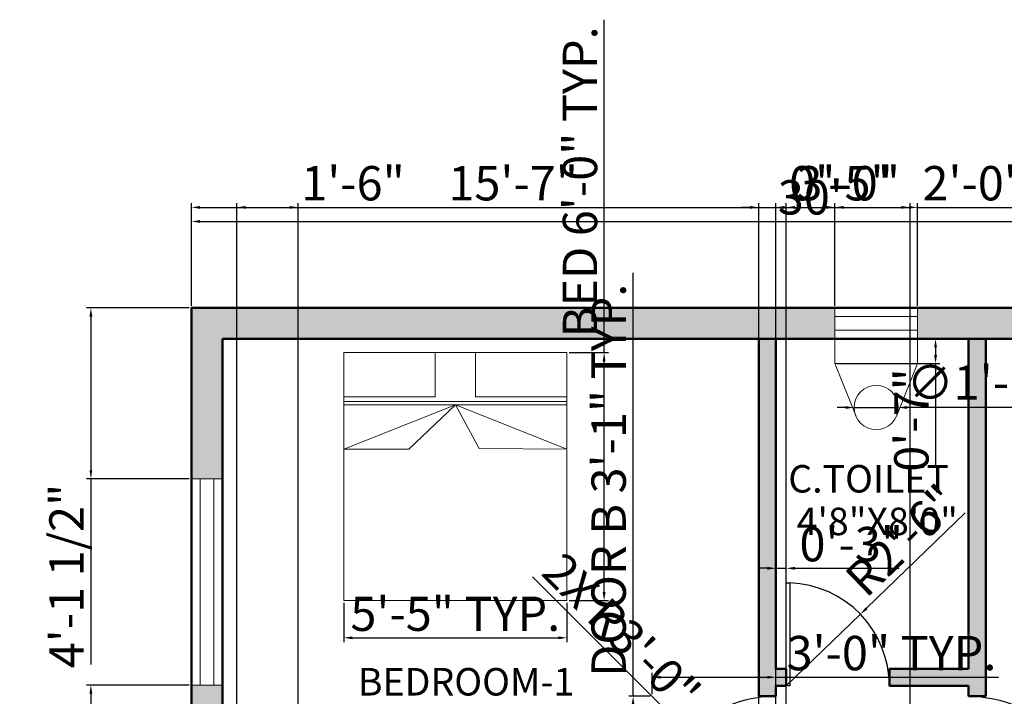
# Model space of a CAD drawing. Units: inches. Extents: x 2719 to 3167, y 1639 to 2327.
# Tile 3 of 4: x 2719 to 3005, y 2130 to 2327. Entities that reach past the tile are written whole.
import ezdxf

# ---------------------------------------------------------------- set-up
doc = ezdxf.new("R2010")
doc.units = ezdxf.units.IN
for name, color, linetype, lineweight in [('A-ANNO-DIMS', 121, 'Continuous', 18), ('A-AREA-IDEN', 121, 'Continuous', 18), ('A-DOOR', 50, 'Continuous', 25), ('A-FLOR-FIXT', 211, 'Continuous', 18), ('A-FURN', 211, 'Continuous', 18), ('A-GLAZ', 191, 'Continuous', 18), ('A-WALL', 7, 'Continuous', 50)]:
    doc.layers.add(name, color=color, linetype=linetype, lineweight=lineweight)
doc.layers.add('A-WALL-PATT', color=251, linetype='Continuous', lineweight=13, true_color=0x636466)
doc.styles.get("Standard").update_dxf_attribs({"font": 'arial.ttf'})
doc.dimstyles.new('ISO-25', dxfattribs={"dimtxt": 10, "dimasz": 2.5, "dimexe": 1.25, "dimexo": 0.625, "dimtad": 1, "dimdec": 0, "dimlunit": 3, "dimtxsty": 'Standard', "dimcen": 2.5, "dimadec": 0, "dimazin": 0, "dimtfac": 1, "dimtdec": 0, "dimtmove": 0, "dimatfit": 3, "dimfxl": 1, "dimarcsym": 0})

# ---------------------------------------------------------------- blocks, each defined once
blk = doc.blocks.new('*D1')
at = {"layer": 'A-ANNO-DIMS', "color": 0, "lineweight": -2, "transparency": 16777216}
for p, q in [((2768.8, 2244.06), (2768.8, 2269.84)), ((2771.3, 2268.59), (3126.3, 2268.59)), ((3128.8, 2244.06), (3128.8, 2269.84))]:
    blk.add_line(p, q, dxfattribs=at)
at = {"layer": 'A-ANNO-DIMS', "color": 0, "transparency": 16777216}
for points in [[(2771.3, 2269.01), (2771.3, 2268.17), (2768.8, 2268.59)], [(3126.3, 2269.01), (3126.3, 2268.17), (3128.8, 2268.59)]]:
    blk.add_solid(points, dxfattribs=at)
at = {"layer": 'Defpoints', "color": 0, "transparency": 16777216}
for p in [(3128.8, 2268.59), (2768.8, 2243.44), (3128.8, 2243.44)]:
    blk.add_point(p, dxfattribs=at)
at = {"layer": 'A-ANNO-DIMS', "color": 0, "transparency": 16777216, "insert": (2948.8, 2274.32), "char_height": 10, "attachment_point": 5}
blk.add_mtext("30'", dxfattribs=at)
blk = doc.blocks.new('BED-DOUBLE')
for p, q in [((0, 57.96), (64.91, 57.96)), ((0, 56.96), (64.91, 56.96)), ((32.46, 56.96), (0, 44.1)), ((32.46, 56.96), (18.94, 44.05)), ((32.46, 56.96), (64.91, 44.04)), ((32.46, 56.96), (39.4, 44.29)), ((18.94, 44.05), (0, 44.05)), ((39.4, 44.29), (64.91, 44.04))]:
    blk.add_line(p, q)
for points in [[(0, 72.15), (64.91, 72.15), (64.91, 0), (0, 0)], [(0, 72.15), (26.55, 72.15), (26.55, 59.27), (0, 59.27)], [(38.37, 72.15), (64.91, 72.15), (64.91, 59.27), (38.37, 59.27)]]:
    blk.add_lwpolyline(points, close=True)
blk = doc.blocks.new('WIN-60IN')
for p, q in [((9, 60), (0, 60)), ((2.5, 60), (2.5, 0)), ((6.5, 60), (6.5, 0)), ((9, 0), (0, 0))]:
    blk.add_line(p, q)
blk = doc.blocks.new('DOOR-36IN-QUARTER-SWING')
for p, q in [((0, 0), (0, 1)), ((0, 1), (36, 1)), ((36, 0), (0, 0)), ((36, 1), (36, 0))]:
    blk.add_line(p, q)
blk.add_arc((36, 1), 36, 90, 180)
blk = doc.blocks.new('*D9')
at = {"layer": 'A-ANNO-DIMS', "color": 0, "lineweight": -2, "transparency": 16777216}
for p, q in [((2888.82, 2230.43), (2888.82, 2327.3)), ((2878.63, 2230.43), (2890.07, 2230.43)), ((2888.82, 2160.78), (2888.82, 2227.93)), ((2878.63, 2158.28), (2890.07, 2158.28))]:
    blk.add_line(p, q, dxfattribs=at)
at = {"layer": 'A-ANNO-DIMS', "color": 0, "transparency": 16777216}
for points in [[(2888.41, 2227.93), (2889.24, 2227.93), (2888.82, 2230.43)], [(2888.41, 2160.78), (2889.24, 2160.78), (2888.82, 2158.28)]]:
    blk.add_solid(points, dxfattribs=at)
at = {"layer": 'Defpoints', "color": 0, "transparency": 16777216}
for p in [(2878, 2230.43), (2888.82, 2230.43), (2878, 2158.28)]:
    blk.add_point(p, dxfattribs=at)
at = {"layer": 'A-ANNO-DIMS', "color": 0, "transparency": 16777216, "insert": (2883.09, 2280.11), "char_height": 10, "attachment_point": 5, "rotation": 90}
blk.add_mtext('BED 6\'-0" TYP.', dxfattribs=at)
blk = doc.blocks.new('*D10')
at = {"layer": 'A-ANNO-DIMS', "color": 0, "lineweight": -2, "transparency": 16777216}
for p, q in [((2813.09, 2157.65), (2813.09, 2146.21)), ((2878, 2157.65), (2878, 2146.21)), ((2815.59, 2147.46), (2875.5, 2147.46))]:
    blk.add_line(p, q, dxfattribs=at)
at = {"layer": 'A-ANNO-DIMS', "color": 0, "transparency": 16777216}
for points in [[(2815.59, 2147.87), (2815.59, 2147.04), (2813.09, 2147.46)], [(2875.5, 2147.87), (2875.5, 2147.04), (2878, 2147.46)]]:
    blk.add_solid(points, dxfattribs=at)
at = {"layer": 'Defpoints', "color": 0, "transparency": 16777216}
for p in [(2813.09, 2158.28), (2878, 2158.28), (2878, 2147.46)]:
    blk.add_point(p, dxfattribs=at)
at = {"layer": 'A-ANNO-DIMS', "color": 0, "transparency": 16777216, "insert": (2845.54, 2153.17), "char_height": 10, "attachment_point": 5}
blk.add_mtext('5\'-5" TYP.', dxfattribs=at)
blk = doc.blocks.new('*D13')
at = {"layer": 'A-ANNO-DIMS', "color": 0, "lineweight": -2, "transparency": 16777216}
for p, q in [((2897.25, 2130.44), (2897.25, 2253.63)), ((2902.17, 2130.44), (2896, 2130.44)), ((2897.25, 2095.94), (2897.25, 2127.94)), ((2902.17, 2093.44), (2896, 2093.44))]:
    blk.add_line(p, q, dxfattribs=at)
at = {"layer": 'A-ANNO-DIMS', "color": 0, "transparency": 16777216}
for points in [[(2896.83, 2127.94), (2897.66, 2127.94), (2897.25, 2130.44)], [(2896.83, 2095.94), (2897.66, 2095.94), (2897.25, 2093.44)]]:
    blk.add_solid(points, dxfattribs=at)
at = {"layer": 'Defpoints', "color": 0, "transparency": 16777216}
for p in [(2897.25, 2130.44), (2902.8, 2130.44), (2902.8, 2093.44)]:
    blk.add_point(p, dxfattribs=at)
at = {"layer": 'A-ANNO-DIMS', "color": 0, "transparency": 16777216, "insert": (2891.44, 2193.29), "char_height": 10, "attachment_point": 5, "rotation": 90}
blk.add_mtext('DOOR B 3\'-1" TYP.', dxfattribs=at)
blk = doc.blocks.new('*D14')
at = {"layer": 'A-ANNO-DIMS', "color": 0, "lineweight": -2, "transparency": 16777216}
for p, q in [((2902.8, 2131.06), (2902.8, 2137.24)), ((2938.8, 2131.06), (2938.8, 2137.24)), ((2905.3, 2135.99), (2936.3, 2135.99)), ((2938.8, 2135.99), (3003.49, 2135.99))]:
    blk.add_line(p, q, dxfattribs=at)
at = {"layer": 'A-ANNO-DIMS', "color": 0, "transparency": 16777216}
for points in [[(2905.3, 2136.4), (2905.3, 2135.57), (2902.8, 2135.99)], [(2936.3, 2136.4), (2936.3, 2135.57), (2938.8, 2135.99)]]:
    blk.add_solid(points, dxfattribs=at)
at = {"layer": 'Defpoints', "color": 0, "transparency": 16777216}
for p in [(2938.8, 2135.99), (2902.8, 2130.44), (2938.8, 2130.44)]:
    blk.add_point(p, dxfattribs=at)
at = {"layer": 'A-ANNO-DIMS', "color": 0, "transparency": 16777216, "insert": (2972.4, 2141.72), "char_height": 10, "attachment_point": 5}
blk.add_mtext('3\'-0" TYP.', dxfattribs=at)
blk = doc.blocks.new('*D17')
at = {"layer": 'A-ANNO-DIMS', "color": 0, "lineweight": -2, "transparency": 16777216}
for p, q in [((2768.8, 2244.06), (2768.8, 2273.94)), ((2955.97, 2244.06), (2955.97, 2273.94)), ((2771.3, 2272.69), (2953.47, 2272.69))]:
    blk.add_line(p, q, dxfattribs=at)
at = {"layer": 'A-ANNO-DIMS', "color": 0, "transparency": 16777216}
for points in [[(2771.3, 2273.1), (2771.3, 2272.27), (2768.8, 2272.69)], [(2953.47, 2273.1), (2953.47, 2272.27), (2955.97, 2272.69)]]:
    blk.add_solid(points, dxfattribs=at)
at = {"layer": 'Defpoints', "color": 0, "transparency": 16777216}
for p in [(2955.97, 2272.69), (2768.8, 2243.44), (2955.97, 2243.44)]:
    blk.add_point(p, dxfattribs=at)
at = {"layer": 'A-ANNO-DIMS', "color": 0, "transparency": 16777216, "insert": (2862.38, 2278.42), "char_height": 10, "attachment_point": 5}
blk.add_mtext('15\'-7"', dxfattribs=at)
blk = doc.blocks.new('*D18')
at = {"layer": 'A-ANNO-DIMS', "color": 0, "lineweight": -2, "transparency": 16777216}
for p, q in [((2955.97, 2244.06), (2955.97, 2273.94)), ((2979.97, 2244.06), (2979.97, 2273.94)), ((2958.47, 2272.69), (2977.47, 2272.69)), ((2979.97, 2272.69), (3010.48, 2272.69))]:
    blk.add_line(p, q, dxfattribs=at)
at = {"layer": 'A-ANNO-DIMS', "color": 0, "transparency": 16777216}
for points in [[(2958.47, 2273.1), (2958.47, 2272.27), (2955.97, 2272.69)], [(2977.47, 2273.1), (2977.47, 2272.27), (2979.97, 2272.69)]]:
    blk.add_solid(points, dxfattribs=at)
at = {"layer": 'Defpoints', "color": 0, "transparency": 16777216}
for p in [(2979.97, 2272.69), (2955.97, 2243.44), (2979.97, 2243.44)]:
    blk.add_point(p, dxfattribs=at)
at = {"layer": 'A-ANNO-DIMS', "color": 0, "transparency": 16777216, "insert": (2996.48, 2278.42), "char_height": 10, "attachment_point": 5}
blk.add_mtext('2\'-0"', dxfattribs=at)
blk = doc.blocks.new('*D19')
at = {"layer": 'A-ANNO-DIMS', "color": 0, "lineweight": -2, "transparency": 16777216}
for p, q in [((2768.17, 2243.44), (2738.3, 2243.44)), ((2739.55, 2240.94), (2739.55, 2196.22)), ((2768.17, 2193.72), (2738.3, 2193.72)), ((2739.55, 2193.72), (2739.55, 2139.68))]:
    blk.add_line(p, q, dxfattribs=at)
at = {"layer": 'A-ANNO-DIMS', "color": 0, "transparency": 16777216}
for points in [[(2739.13, 2240.94), (2739.96, 2240.94), (2739.55, 2243.44)], [(2739.13, 2196.22), (2739.96, 2196.22), (2739.55, 2193.72)]]:
    blk.add_solid(points, dxfattribs=at)
at = {"layer": 'Defpoints', "color": 0, "transparency": 16777216}
for p in [(2768.8, 2243.44), (2739.55, 2193.72), (2768.8, 2193.72)]:
    blk.add_point(p, dxfattribs=at)
at = {"layer": 'A-ANNO-DIMS', "color": 0, "transparency": 16777216, "insert": (2733.75, 2165.45), "char_height": 10, "attachment_point": 5, "rotation": 90}
blk.add_mtext('4\'-1 1/2"', dxfattribs=at)
blk = doc.blocks.new('*D20')
at = {"layer": 'A-ANNO-DIMS', "color": 0, "lineweight": -2, "transparency": 16777216}
for p, q in [((2768.17, 2133.72), (2738.3, 2133.72)), ((2739.55, 2131.22), (2739.55, 2064.55)), ((2768.17, 2062.05), (2738.3, 2062.05))]:
    blk.add_line(p, q, dxfattribs=at)
at = {"layer": 'A-ANNO-DIMS', "color": 0, "transparency": 16777216}
for points in [[(2739.13, 2131.22), (2739.96, 2131.22), (2739.55, 2133.72)], [(2739.13, 2064.55), (2739.96, 2064.55), (2739.55, 2062.05)]]:
    blk.add_solid(points, dxfattribs=at)
at = {"layer": 'Defpoints', "color": 0, "transparency": 16777216}
for p in [(2768.8, 2133.72), (2739.55, 2062.05), (2768.8, 2062.05)]:
    blk.add_point(p, dxfattribs=at)
at = {"layer": 'A-ANNO-DIMS', "color": 0, "transparency": 16777216, "insert": (2733.75, 2097.88), "char_height": 10, "attachment_point": 5, "rotation": 90}
blk.add_mtext('5\'-11 1/2"', dxfattribs=at)
blk = doc.blocks.new('*D28')
at = {"layer": 'A-ANNO-DIMS', "color": 0, "lineweight": -2, "transparency": 16777216}
for p, q in [((2933.8, 2041.15), (2933.8, 2273.94)), ((2938.8, 2041.15), (2938.8, 2273.94)), ((2931.3, 2272.69), (2928.8, 2272.69)), ((2933.8, 2272.69), (2938.8, 2272.69)), ((2941.3, 2272.69), (2971.63, 2272.69))]:
    blk.add_line(p, q, dxfattribs=at)
at = {"layer": 'A-ANNO-DIMS', "color": 0, "transparency": 16777216}
for points in [[(2931.3, 2273.1), (2931.3, 2272.27), (2933.8, 2272.69)], [(2941.3, 2273.1), (2941.3, 2272.27), (2938.8, 2272.69)]]:
    blk.add_solid(points, dxfattribs=at)
at = {"layer": 'Defpoints', "color": 0, "transparency": 16777216}
for p in [(2938.8, 2272.69), (2933.8, 2040.53), (2938.8, 2040.53)]:
    blk.add_point(p, dxfattribs=at)
at = {"layer": 'A-ANNO-DIMS', "color": 0, "transparency": 16777216, "insert": (2957.71, 2278.42), "char_height": 10, "attachment_point": 5}
blk.add_mtext('0\'-5"', dxfattribs=at)
blk = doc.blocks.new('*D33')
at = {"layer": 'A-ANNO-DIMS', "color": 0, "lineweight": -2, "transparency": 16777216}
for p, q in [((2782.04, 2038.37), (2782.04, 2273.94)), ((2799.85, 2038.37), (2799.85, 2273.94)), ((2784.54, 2272.69), (2797.35, 2272.69)), ((2799.85, 2272.69), (2829.24, 2272.69))]:
    blk.add_line(p, q, dxfattribs=at)
at = {"layer": 'A-ANNO-DIMS', "color": 0, "transparency": 16777216}
for points in [[(2784.54, 2273.1), (2784.54, 2272.27), (2782.04, 2272.69)], [(2797.35, 2273.1), (2797.35, 2272.27), (2799.85, 2272.69)]]:
    blk.add_solid(points, dxfattribs=at)
at = {"layer": 'Defpoints', "color": 0, "transparency": 16777216}
for p in [(2799.85, 2272.69), (2782.04, 2037.74), (2799.85, 2037.74)]:
    blk.add_point(p, dxfattribs=at)
at = {"layer": 'A-ANNO-DIMS', "color": 0, "transparency": 16777216, "insert": (2815.79, 2278.42), "char_height": 10, "attachment_point": 5}
blk.add_mtext('1\'-6"', dxfattribs=at)
blk = doc.blocks.new('*D48')
at = {"layer": 'A-ANNO-DIMS', "color": 0, "lineweight": -2, "transparency": 16777216}
for p, q in [((2941.8, 1796.06), (2941.8, 2273.94)), ((2977.8, 1796.06), (2977.8, 2273.94)), ((2944.3, 2272.69), (2975.3, 2272.69))]:
    blk.add_line(p, q, dxfattribs=at)
at = {"layer": 'A-ANNO-DIMS', "color": 0, "transparency": 16777216}
for points in [[(2944.3, 2273.1), (2944.3, 2272.27), (2941.8, 2272.69)], [(2975.3, 2273.1), (2975.3, 2272.27), (2977.8, 2272.69)]]:
    blk.add_solid(points, dxfattribs=at)
at = {"layer": 'Defpoints', "color": 0, "transparency": 16777216}
for p in [(2977.8, 2272.69), (2941.8, 1795.44), (2977.8, 1795.44)]:
    blk.add_point(p, dxfattribs=at)
at = {"layer": 'A-ANNO-DIMS', "color": 0, "transparency": 16777216, "insert": (2959.8, 2278.42), "char_height": 10, "attachment_point": 5}
blk.add_mtext('3\'-0"', dxfattribs=at)
blk = doc.blocks.new('*D51')
at = {"layer": 'A-ANNO-DIMS', "color": 0, "lineweight": -2, "transparency": 16777216}
for p, q in [((2938.8, 2139.06), (2938.8, 2168.94)), ((2941.8, 2139.06), (2941.8, 2168.94)), ((2936.3, 2167.69), (2933.8, 2167.69)), ((2938.8, 2167.69), (2941.8, 2167.69)), ((2944.3, 2167.69), (2974.63, 2167.69))]:
    blk.add_line(p, q, dxfattribs=at)
at = {"layer": 'A-ANNO-DIMS', "color": 0, "transparency": 16777216}
for points in [[(2936.3, 2168.1), (2936.3, 2167.27), (2938.8, 2167.69)], [(2944.3, 2168.1), (2944.3, 2167.27), (2941.8, 2167.69)]]:
    blk.add_solid(points, dxfattribs=at)
at = {"layer": 'Defpoints', "color": 0, "transparency": 16777216}
for p in [(2941.8, 2167.69), (2938.8, 2138.44), (2941.8, 2138.44)]:
    blk.add_point(p, dxfattribs=at)
at = {"layer": 'A-ANNO-DIMS', "color": 0, "transparency": 16777216, "insert": (2960.71, 2173.42), "char_height": 10, "attachment_point": 5}
blk.add_mtext('0\'-3"', dxfattribs=at)
blk = doc.blocks.new('*D52')
at = {"layer": 'A-ANNO-DIMS', "color": 0, "lineweight": -2, "transparency": 16777216}
for p, q in [((2956.6, 2234.44), (2986.47, 2234.44)), ((2985.22, 2231.94), (2985.22, 2229.75)), ((2956.6, 2227.25), (2986.47, 2227.25)), ((2985.22, 2227.25), (2985.22, 2196.91))]:
    blk.add_line(p, q, dxfattribs=at)
at = {"layer": 'A-ANNO-DIMS', "color": 0, "transparency": 16777216}
for points in [[(2984.81, 2231.94), (2985.64, 2231.94), (2985.22, 2234.44)], [(2984.81, 2229.75), (2985.64, 2229.75), (2985.22, 2227.25)]]:
    blk.add_solid(points, dxfattribs=at)
at = {"layer": 'Defpoints', "color": 0, "transparency": 16777216}
for p in [(2955.97, 2234.44), (2955.97, 2227.25), (2985.22, 2227.25)]:
    blk.add_point(p, dxfattribs=at)
at = {"layer": 'A-ANNO-DIMS', "color": 0, "transparency": 16777216, "insert": (2979.49, 2210.83), "char_height": 10, "attachment_point": 5, "rotation": 90}
blk.add_mtext('0\'-7"', dxfattribs=at)
blk = doc.blocks.new('*D54')
at = {"layer": 'A-ANNO-DIMS', "color": 0, "lineweight": -2, "transparency": 16777216}
for p, q in [((2868.04, 2165.19), (2911.57, 2121.66)), ((2938.8, 2094.44), (2913.34, 2119.89))]:
    blk.add_line(p, q, dxfattribs=at)
at = {"layer": 'A-ANNO-DIMS', "color": 0, "transparency": 16777216}
blk.add_solid([(2911.87, 2121.96), (2911.28, 2121.37), (2913.34, 2119.89)], dxfattribs=at)
at = {"layer": 'Defpoints', "color": 0, "transparency": 16777216}
for p in [(2913.34, 2119.89), (2938.8, 2094.44)]:
    blk.add_point(p, dxfattribs=at)
at = {"layer": 'A-ANNO-DIMS', "color": 0, "transparency": 16777216, "insert": (2892.98, 2148.36), "char_height": 10, "attachment_point": 5, "rotation": 315.0006}
blk.add_mtext('2X R3\'-0"', dxfattribs=at)
blk = doc.blocks.new('*D55')
at = {"layer": 'A-ANNO-DIMS', "color": 0, "lineweight": -2, "transparency": 16777216}
for p, q in [((2993.85, 2183.78), (2965.16, 2156.04)), ((2941.8, 2133.45), (2963.37, 2154.3))]:
    blk.add_line(p, q, dxfattribs=at)
at = {"layer": 'A-ANNO-DIMS', "color": 0, "transparency": 16777216}
blk.add_solid([(2964.87, 2156.34), (2965.45, 2155.74), (2963.37, 2154.3)], dxfattribs=at)
at = {"layer": 'Defpoints', "color": 0, "transparency": 16777216}
for p in [(2963.37, 2154.3), (2941.8, 2133.45)]:
    blk.add_point(p, dxfattribs=at)
at = {"layer": 'A-ANNO-DIMS', "color": 0, "transparency": 16777216, "insert": (2976.42, 2174.9), "char_height": 10, "attachment_point": 5, "rotation": 44.029}
blk.add_mtext('R2\'-6"', dxfattribs=at)
blk = doc.blocks.new('*D57')
at = {"layer": 'A-ANNO-DIMS', "color": 0, "lineweight": -2, "transparency": 16777216}
for p, q in [((2959.06, 2214.46), (2956.56, 2214.46)), ((2961.56, 2214.46), (2974.39, 2214.46)), ((3018.1, 2214.46), (2976.89, 2214.46))]:
    blk.add_line(p, q, dxfattribs=at)
at = {"layer": 'A-ANNO-DIMS', "color": 0, "transparency": 16777216}
for points in [[(2959.06, 2214.88), (2959.06, 2214.05), (2961.56, 2214.46)], [(2976.89, 2214.88), (2976.89, 2214.05), (2974.39, 2214.46)]]:
    blk.add_solid(points, dxfattribs=at)
at = {"layer": 'Defpoints', "color": 0, "transparency": 16777216}
for p in [(2961.56, 2214.46), (2974.39, 2214.46)]:
    blk.add_point(p, dxfattribs=at)
at = {"layer": 'A-ANNO-DIMS', "color": 0, "transparency": 16777216, "insert": (2998.74, 2220.47), "char_height": 10, "attachment_point": 5, "rotation": 359.9976}
blk.add_mtext('∅1\'-1"', dxfattribs=at)

msp = doc.modelspace()

# ---------------------------------------------------------------- hatches: boundary and pattern name
at = {"layer": 'A-WALL-PATT'}
h = msp.add_hatch(color=256, dxfattribs=at)
h.dxf.hatch_style = 1
h.paths.add_polyline_path([(2955.97, 2243.44), (2768.8, 2243.44), (2768.8, 2193.72), (2777.8, 2193.72), (2777.8, 2234.44), (2955.97, 2234.44)])
h = msp.add_hatch(color=256, dxfattribs=at)
h.dxf.hatch_style = 1
h.paths.add_polyline_path([(3128.8, 2243.44), (2979.97, 2243.44), (2979.97, 2234.44), (3119.8, 2234.44), (3119.8, 2196.72), (3128.8, 2196.72)])
h = msp.add_hatch(color=256, dxfattribs=at)
h.dxf.hatch_style = 1
h.paths.add_polyline_path([(2941.8, 2138.44), (2938.8, 2138.44), (2938.8, 2234.44), (2933.8, 2234.44), (2933.8, 2133.44), (2933.8, 2130.44), (2938.8, 2130.44), (2938.8, 2133.44), (2941.8, 2133.44)])
h = msp.add_hatch(color=256, dxfattribs=at)
h.dxf.hatch_style = 1
h.paths.add_polyline_path([(2999.8, 2234.44), (2994.8, 2234.44), (2994.8, 2138.44), (2971.8, 2138.44), (2971.8, 2133.44), (2994.8, 2133.44), (2994.8, 2130.44), (2999.8, 2130.44), (2999.8, 2133.44)])
h = msp.add_hatch(color=256, dxfattribs=at)
h.dxf.hatch_style = 1
h.paths.add_polyline_path([(2777.8, 2133.72), (2768.8, 2133.72), (2768.8, 2062.05), (2777.8, 2062.05)])

# ---------------------------------------------------------------- linework, layer by layer
at = {"layer": 'A-DOOR'}
for p, q in [((2941.8, 2133.44), (2941.8, 2163.44)), ((2941.8, 2163.44), (2942.8, 2163.44)), ((2942.8, 2163.44), (2942.8, 2133.44)), ((2942.8, 2133.44), (2941.8, 2133.44))]:
    msp.add_line(p, q, dxfattribs=at)
msp.add_arc((2941.8, 2133.45), 30, 359.9682, 88.0898, dxfattribs=at)
at = {"layer": 'A-FLOR-FIXT'}
for p, q in [((2955.97, 2227.25), (2962.02, 2212.09)), ((2979.97, 2227.25), (2973.93, 2212.09))]:
    msp.add_line(p, q, dxfattribs=at)
msp.add_lwpolyline([(2955.97, 2234.44), (2979.97, 2234.44), (2979.97, 2227.25), (2955.97, 2227.25)], close=True, dxfattribs=at)
msp.add_circle((2967.97, 2214.46), 6.41, dxfattribs=at)
at = {"layer": 'A-GLAZ'}
for p, q in [((2955.97, 2243.44), (2955.97, 2234.44)), ((2979.97, 2243.44), (2979.97, 2234.44)), ((2955.97, 2240.94), (2979.97, 2240.94)), ((2955.97, 2236.94), (2979.97, 2236.94))]:
    msp.add_line(p, q, dxfattribs=at)
at = {"layer": 'A-WALL'}
for p, q in [((2777.8, 2234.44), (3119.8, 2234.44)), ((2777.8, 1712.44), (2777.8, 2234.44)), ((2933.8, 2133.44), (2933.8, 2234.44)), ((2938.8, 2138.44), (2938.8, 2234.44)), ((2994.8, 2138.44), (2994.8, 2234.44)), ((2999.8, 2133.44), (2999.8, 2234.44)), ((2938.8, 2138.44), (2941.8, 2138.44)), ((2941.8, 2138.44), (2941.8, 2133.44)), ((2971.8, 2138.44), (2971.8, 2133.44)), ((2971.8, 2138.44), (2994.8, 2138.44)), ((2933.8, 2130.44), (2933.8, 2133.44)), ((2938.8, 2133.44), (2941.8, 2133.44)), ((2938.8, 2133.44), (2938.8, 2130.44)), ((2971.8, 2133.44), (2994.8, 2133.44)), ((2994.8, 2130.44), (2994.8, 2133.44)), ((2999.8, 2133.44), (2999.8, 2130.44)), ((2938.8, 2130.44), (2933.8, 2130.44)), ((2999.8, 2130.44), (2994.8, 2130.44))]:
    msp.add_line(p, q, dxfattribs=at)
msp.add_lwpolyline([(2941.8, 1703.44), (2768.8, 1703.44), (2768.8, 2243.44), (3128.8, 2243.44), (3128.8, 1703.44), (2989.8, 1703.44)], dxfattribs=at)

# ---------------------------------------------------------------- block references
at = {"layer": 'A-DOOR'}
msp.add_blockref('DOOR-36IN-QUARTER-SWING', (2902.8, 2093.44), dxfattribs=at)
at = {"layer": 'A-DOOR', "extrusion": (0, 0, -1), "zscale": -1}
msp.add_blockref('DOOR-36IN-QUARTER-SWING', (-3030.8, 2093.44), dxfattribs=at)
at = {"layer": 'A-FURN'}
msp.add_blockref('BED-DOUBLE', (2813.09, 2158.28), dxfattribs=at)
at = {"layer": 'A-GLAZ'}
msp.add_blockref('WIN-60IN', (2768.8, 2133.72), dxfattribs=at)

# ---------------------------------------------------------------- texts
at = {"layer": 'A-AREA-IDEN'}
for tag, p in [('C.TOILET', (2942.38, 2189.72)), ('4\'8"X8\'0"', (2944.83, 2177.33)), ('BEDROOM-1', (2817.21, 2130.67))]:
    msp.add_attdef(tag, p, '', height=8, dxfattribs=at)

# ---------------------------------------------------------------- dimensions: what is measured, and where the dimension line sits
at = {"layer": 'A-ANNO-DIMS'}
for base, p1, p2, text, picture, middle in [((2888.8241, 2230.4299), (2878.0015, 2158.2792), (2878.0015, 2230.4299), 'BED <> TYP.', '*D9', (2883.0933, 2280.1135)), ((2897.25, 2130.44), (2902.8, 2093.44), (2902.8, 2130.44), 'DOOR B <> TYP.', '*D13', (2891.44, 2193.29))]:
    dim = msp.add_linear_dim(base=base, p1=p1, p2=p2, angle=90, text=text, dimstyle='ISO-25', override={"dimdec": 1, "dimlfac": 1, "dimrnd": 0, "dimzin": 1, "dimdsep": 46, "dimlunit": 4, "dimfrac": 2}, dxfattribs=at)
    dim.commit()
    dim.dimension.update_dxf_attribs({"geometry": picture, "text_midpoint": middle})
for base, p1, p2, override, picture, middle in [((2955.97, 2272.69), (2768.8, 2243.44), (2955.97, 2243.44), {"dimdec": 1, "dimlfac": 1, "dimrnd": 0, "dimzin": 1, "dimdsep": 46, "dimlunit": 4, "dimfrac": 2}, '*D17', (2862.38, 2278.42)), ((2799.85, 2272.69), (2782.04, 2037.74), (2799.85, 2037.74), {"dimdec": 1, "dimlfac": 1, "dimrnd": 0, "dimzin": 1, "dimdsep": 46, "dimlunit": 4, "dimfrac": 2}, '*D33', (2815.79, 2278.42)), ((2938.8, 2272.69), (2933.8, 2040.53), (2938.8, 2040.53), {"dimdec": 1, "dimlfac": 1, "dimrnd": 0, "dimzin": 1, "dimdsep": 46, "dimlunit": 4, "dimfrac": 2}, '*D28', (2957.71, 2278.42)), ((2977.8, 2272.69), (2941.8, 1795.44), (2977.8, 1795.44), {"dimdec": 1, "dimlfac": 1, "dimrnd": 0, "dimzin": 1, "dimdsep": 46, "dimlunit": 4, "dimfrac": 2}, '*D48', (2959.8, 2278.42)), ((2979.97, 2272.69), (2955.97, 2243.44), (2979.97, 2243.44), {"dimdec": 1, "dimlfac": 1, "dimrnd": 0, "dimzin": 1, "dimdsep": 46, "dimlunit": 4, "dimfrac": 2}, '*D18', (2996.48, 2278.42)), ((3128.8, 2268.59), (2768.8, 2243.44), (3128.8, 2243.44), {"dimclrd": 0, "dimclre": 0, "dimclrt": 0}, '*D1', (2948.8, 2274.32)), ((2941.8, 2167.69), (2938.8, 2138.44), (2941.8, 2138.44), {"dimdec": 1, "dimlfac": 1, "dimrnd": 0, "dimzin": 1, "dimdsep": 46, "dimlunit": 4, "dimfrac": 2}, '*D51', (2960.71, 2173.42))]:
    dim = msp.add_linear_dim(base=base, p1=p1, p2=p2, dimstyle='ISO-25', override=override, dxfattribs=at)
    dim.commit()
    dim.dimension.update_dxf_attribs({"geometry": picture, "text_midpoint": middle})
for base, p1, p2, angle, picture, middle in [((2739.55, 2193.72), (2768.8, 2243.44), (2768.8, 2193.72), 90, '*D19', (2733.75, 2165.45)), ((2985.22, 2227.25), (2955.97, 2234.44), (2955.97, 2227.25), 270, '*D52', (2979.49, 2210.83)), ((2739.55, 2062.05), (2768.8, 2133.72), (2768.8, 2062.05), 90, '*D20', (2733.75, 2097.88))]:
    dim = msp.add_linear_dim(base=base, p1=p1, p2=p2, angle=angle, dimstyle='ISO-25', override={"dimdec": 1, "dimlfac": 1, "dimrnd": 0, "dimzin": 1, "dimdsep": 46, "dimlunit": 4, "dimfrac": 2}, dxfattribs=at)
    dim.commit()
    dim.dimension.update_dxf_attribs({"geometry": picture, "text_midpoint": middle})
dim = msp.add_diameter_dim_2p(p1=(2961.56, 2214.46), p2=(2974.39, 2214.46), dimstyle='ISO-25', override={"dimdec": 1, "dimlfac": 1, "dimrnd": 0, "dimzin": 1, "dimdsep": 46, "dimlunit": 4, "dimfrac": 2}, dxfattribs=at)
dim.commit()
dim.dimension.update_dxf_attribs({"geometry": '*D57', "text_midpoint": (2998.74, 2214.46)})
dim = msp.add_radius_dim(center=(2941.8, 2133.45), mpoint=(2963.37, 2154.3), dimstyle='ISO-25', override={"dimdec": 1, "dimlfac": 1, "dimrnd": 0, "dimzin": 1, "dimdsep": 46, "dimlunit": 4, "dimfrac": 2}, dxfattribs=at)
dim.commit()
dim.dimension.update_dxf_attribs({"geometry": '*D55', "text_midpoint": (2976.42, 2174.9)})
dim = msp.add_radius_dim(center=(2938.8, 2094.44), mpoint=(2913.34, 2119.89), text='2X <>', dimstyle='ISO-25', override={"dimdec": 1, "dimlfac": 1, "dimrnd": 0, "dimzin": 1, "dimdsep": 46, "dimlunit": 4, "dimfrac": 2}, dxfattribs=at)
dim.commit()
dim.dimension.update_dxf_attribs({"geometry": '*D54', "text_midpoint": (2892.98, 2148.36)})
for base, p1, p2, picture, middle in [((2878, 2147.46), (2813.09, 2158.28), (2878, 2158.28), '*D10', (2845.54, 2153.17)), ((2938.8, 2135.99), (2902.8, 2130.44), (2938.8, 2130.44), '*D14', (2972.4, 2141.72))]:
    dim = msp.add_linear_dim(base=base, p1=p1, p2=p2, text='<> TYP.', dimstyle='ISO-25', override={"dimdec": 1, "dimlfac": 1, "dimrnd": 0, "dimzin": 1, "dimdsep": 46, "dimlunit": 4, "dimfrac": 2}, dxfattribs=at)
    dim.commit()
    dim.dimension.update_dxf_attribs({"geometry": picture, "text_midpoint": middle})

doc.saveas('drawing.dxf')
